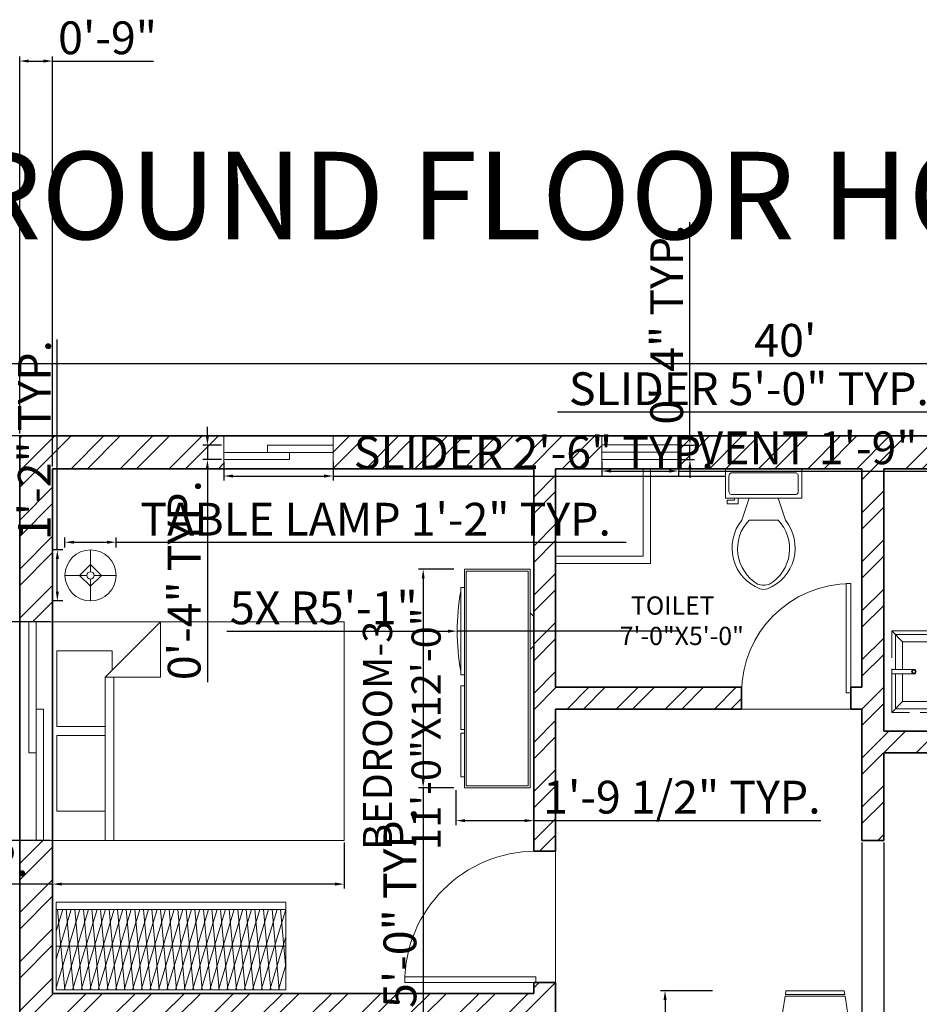
# Model space of a CAD drawing. Units: inches. Extents: x 889 to 1572, y 7262 to 8387.
# Tile 6 of 8: x 1016 to 1263, y 8117 to 8387. Entities that reach past the tile are written whole.
import ezdxf

# ---------------------------------------------------------------- set-up
doc = ezdxf.new("R2010")
doc.units = ezdxf.units.IN
doc.linetypes.add('ACAD_ISO02W100', pattern=[15, 12, -3])
for name, color, linetype, lineweight in [('A-ANNO-DIMS', 2, 'Continuous', 18), ('A-ANNO-TITL', 7, 'Continuous', 35), ('A-AREA-IDEN', 7, 'Continuous', 18), ('A-DOOR', 4, 'Continuous', 18), ('A-FIXT-HIDN', 9, 'ACAD_ISO02W100', 13), ('A-FLOR-FIXT', 9, 'Continuous', 18), ('A-FURN', 8, 'Continuous', 18), ('A-FURN-PATT', 252, 'Continuous', 13), ('A-WALL', 7, 'Continuous', 35), ('A-WALL-PATT', 252, 'Continuous', 13), ('C-SITE', 7, 'Continuous', 30)]:
    doc.layers.add(name, color=color, linetype=linetype, lineweight=lineweight)
doc.layers.add('A-GLAZ', color=244, linetype='Continuous', lineweight=18, true_color=0x991b1e)
doc.styles.get("Standard").update_dxf_attribs({"font": 'arial.ttf'})
doc.dimstyles.new('ISO-25', dxfattribs={"dimtxt": 9, "dimasz": 2.5, "dimexe": 1.25, "dimexo": 0.625, "dimtad": 1, "dimlunit": 3, "dimtxsty": 'Standard', "dimcen": 2.5, "dimadec": 0, "dimazin": 0, "dimtfac": 1, "dimtmove": 0, "dimatfit": 3, "dimfxl": 1, "dimarcsym": 0})

# ---------------------------------------------------------------- blocks, each defined once
blk = doc.blocks.new('*U5')
for p, q in [((-40, 0), (-40, 6)), ((0, 0), (0, 6))]:
    blk.add_line(p, q)
blk.add_lwpolyline([(0, 0), (0, -40), (-1.75, -40), (-1.75, 0)], close=True)
blk.add_arc((0, 0), 40, 180, 270)
blk = doc.blocks.new('*U6')
for p, q in [((0, 0), (0, 6)), ((40, 0), (40, 6))]:
    blk.add_line(p, q)
blk.add_lwpolyline([(0, 0), (0, -40), (1.75, -40), (1.75, 0)], close=True)
blk.add_arc((0, 0), 40, 270, 360)
blk = doc.blocks.new('*U10')
for p, q in [((9.5, -6), (9.5, -2)), ((-8, -8.5), (-8, -8)), ((-7, -8), (-7, -9.5)), ((-4, -8), (-6, -14)), ((4, -8), (6, -14)), ((-10, -8.5), (-8, -8.5)), ((-10, -9.5), (-10, -8.5)), ((-7, -9.5), (-10, -9.5)), ((4, -14), (-4, -14))]:
    blk.add_line(p, q)
blk.add_lwpolyline([(10.5, -8), (10.5, 0), (-10.5, 0), (-10.5, -8)], close=True)
for points in [[(-9.5, -2), (-9.5, -6)], [(8.5, -1), (-8.5, -1)], [(-8.5, -7), (8.5, -7)]]:
    blk.add_lwpolyline(points)
for centre, radius, start, end in [((-8.62, -1.88), 0.884, 81.8699, 188.1301), ((8.62, -1.88), 0.884, 351.8699, 98.1301), ((-8.62, -6.12), 0.884, 171.8699, 278.1301), ((8.62, -6.12), 0.884, 261.8699, 8.1301), ((3.52, -21.58), 12.17, 141.4691, 247.9714), ((4.2, -21.82), 11.33, 136.3677, 238.9468), ((-3.52, -21.58), 12.17, 292.0284, 38.5307), ((-4.2, -21.82), 11.33, 301.053, 43.6321), ((0, -27.88), 4, 245.7318, 294.2682), ((0, -29), 4, 254.8605, 285.1395)]:
    blk.add_arc(centre, radius, start, end)
blk = doc.blocks.new('Bed - Queen')
for p, q in [((0, -80.00003), (0, 0)), ((0, 0), (59.99999, 0)), ((59.99999, 0), (59.99999, -80.00003)), ((7.99999, -1.2), (28.79998, -1.2)), ((7.99999, -14.4), (7.99999, -1.2)), ((28.79998, -1.2), (28.79998, -14.4)), ((31.19999, -1.2), (51.99999, -1.2)), ((31.19999, -14.4), (31.19999, -1.2)), ((51.99999, -1.2), (51.99999, -16.4)), ((0, -14.4), (44.8, -14.4)), ((59.99999, -29.6), (44.8, -14.4)), ((44.8, -14.4), (44.8, -29.6)), ((44.8, -16.8), (0, -16.8)), ((51.99999, -16.4), (46.79936, -16.4)), ((44.8, -29.6), (59.99999, -29.6)), ((59.99999, -80.00003), (0, -80.00003))]:
    blk.add_line(p, q)
blk = doc.blocks.new('Entertainment Center')
for p, q in [((-4, 0), (-5, -1)), ((4, 0), (-4, 0)), ((5, -1), (4, 0)), ((-17, -19), (-17, -1)), ((-17, -1), (43, -1)), ((-16.5, -18.5), (-16.5, -1.5)), ((-16.5, -1.5), (42.5, -1.5)), ((42.5, -1.5), (42.5, -18.5)), ((43, -1), (43, -19)), ((42.5, -18.5), (-16.5, -18.5)), ((43, -19), (-17, -19)), ((-12, -20), (-12, -19)), ((12, -20), (-12, -20)), ((12, -19), (12, -20)), ((15, -20), (15, -19)), ((27, -20), (15, -20)), ((27, -19), (27, -20)), ((28, -20), (28, -19)), ((40, -20), (28, -20)), ((40, -19), (40, -20))]:
    blk.add_line(p, q)
blk.add_arc((0, 40), 61, 259.6111, 280.3889)
blk = doc.blocks.new('Dining Set - 36 x 72 in.')
for p, q in [((-22, 27.5), (-22.1562, 26.50042)), ((-22, 27.5), (-6, 27.5)), ((-5.8437, 26.49966), (-6, 27.5)), ((6, 27.5), (5.8438, 26.50042)), ((6, 27.5), (22, 27.5)), ((22.1563, 26.49966), (22, 27.5)), ((-22.2343, 26.00059), (-23.4847, 17.99762)), ((-22.2304, 26), (-5.7608, 26)), ((-5.8416, 26.5), (-22.1534, 26.5)), ((-4.5152, 17.99762), (-5.7655, 25.99926)), ((5.7657, 26.00059), (4.5153, 17.99762)), ((5.7696, 26), (22.2392, 26)), ((22.1584, 26.5), (5.8466, 26.5)), ((23.4848, 17.99762), (22.2345, 25.99926)), ((36, 18), (-36, 18)), ((-36, 18), (-36, -18)), ((36, -18), (36, 18)), ((-45.5, 8), (-44.5004, 8.15617)), ((-44.5, -8.15843), (-44.5, 8.15338)), ((-44.0006, 8.23428), (-35.9976, 9.48474)), ((-44, 8.23041), (-44, -8.23915)), ((44.0006, 8.23428), (35.9976, 9.48474)), ((44, 8.23041), (44, -8.23915)), ((44.5, -8.15843), (44.5, 8.15338)), ((45.5, 8), (44.5005, 8.15617)), ((-45.5, 8), (-45.5, -8)), ((45.5, 8), (45.5, -8)), ((-44.4997, -8.15631), (-45.5, -8)), ((44.4997, -8.15631), (45.5, -8)), ((-35.9976, -9.48476), (-43.9993, -8.2345)), ((35.9976, -9.48476), (43.9993, -8.2345)), ((-36, -18), (36, -18)), ((-22.2343, -26.0006), (-23.4847, -17.99762)), ((-4.5152, -17.99762), (-5.7655, -25.99928)), ((5.7657, -26.0006), (4.5153, -17.99762)), ((23.4848, -17.99762), (22.2345, -25.99928)), ((-22.2304, -26), (-5.7608, -26)), ((-22, -27.5), (-22.1562, -26.50044)), ((-5.8416, -26.5), (-22.1534, -26.5)), ((-5.8437, -26.49967), (-6, -27.5)), ((5.7696, -26), (22.2392, -26)), ((6, -27.5), (5.8438, -26.50044)), ((22.1584, -26.5), (5.8466, -26.5)), ((22.1563, -26.49967), (22, -27.5)), ((-22, -27.5), (-6, -27.5)), ((6, -27.5), (22, -27.5))]:
    blk.add_line(p, q)
for points in [[(-36, 15), (-31.1772, 14.97754), (-26.8079, 14.91406), (-22.8538, 14.81543), (-19.276, 14.6875), (-16.0362, 14.53613), (-13.0957, 14.36718), (-10.4159, 14.18652), (-7.9583, 14), (-5.6904, 13.81315), (-3.6035, 13.63021), (-1.6954, 13.45508), (0.0365, 13.29166), (1.5945, 13.14388), (2.9811, 13.01562), (4.1988, 12.9108), (5.25, 12.83333), (6.1393, 12.78613), (6.8802, 12.76823), (7.4883, 12.77767), (7.9792, 12.8125), (8.3685, 12.87077), (8.6719, 12.95052), (8.9049, 13.0498), (9.0833, 13.16666), (9.2205, 13.29899), (9.3216, 13.44401), (9.3895, 13.59879), (9.4271, 13.76041), (9.4373, 13.92594), (9.4232, 14.09245), (9.3875, 14.257), (9.3333, 14.41666), (9.2638, 14.56917), (9.1836, 14.71484), (9.0975, 14.85465), (9.0104, 14.98958), (8.9272, 15.1206), (8.8529, 15.2487), (8.7922, 15.37483), (8.75, 15.5), (8.7305, 15.62467), (8.7344, 15.74739), (8.7617, 15.86621), (8.8125, 15.97916), (8.8867, 16.08431), (8.9844, 16.17968), (9.1055, 16.26334), (9.25, 16.33333), (9.4189, 16.38802), (9.6172, 16.42708), (9.8506, 16.45052), (10.125, 16.45833), (10.4463, 16.45052), (10.8203, 16.42708), (11.2529, 16.38802), (11.75, 16.33333), (12.3184, 16.26318), (12.9694, 16.17838), (13.7151, 16.07991), (14.5677, 15.96875), (15.5395, 15.84586), (16.6426, 15.71224), (17.8893, 15.56884), (19.2917, 15.41666), (20.859, 15.25667), (22.5879, 15.08984), (24.4721, 14.91715), (26.5052, 14.73958), (28.6809, 14.5581), (30.9929, 14.3737), (33.4347, 14.18733), (36, 14)], [(-36, 10), (-28.9766, 10.14274), (-23.1725, 10.20442), (-18.4241, 10.19775), (-14.5677, 10.13541), (-11.4399, 10.03011), (-8.877, 9.89453), (-6.7154, 9.74137), (-4.7917, 9.58333), (-2.9698, 9.43082), (-1.2246, 9.28515), (0.4415, 9.14534), (2.026, 9.01041), (3.5266, 8.87939), (4.9408, 8.7513), (6.266, 8.62516), (7.5, 8.5), (8.6411, 8.37549), (9.6914, 8.2539), (10.6538, 8.13818), (11.5312, 8.03125), (12.3267, 7.93603), (13.043, 7.85547), (13.6831, 7.79248), (14.25, 7.75), (14.7471, 7.7303), (15.1797, 7.73307), (15.5537, 7.75732), (15.875, 7.80208), (16.1494, 7.86637), (16.3828, 7.94922), (16.5811, 8.04964), (16.75, 8.16666), (16.8944, 8.29915), (17.0143, 8.44531), (17.1089, 8.60319), (17.1771, 8.77083), (17.218, 8.94629), (17.2305, 9.1276), (17.2137, 9.31282), (17.1667, 9.5), (17.0895, 9.6875), (16.987, 9.875), (16.8649, 10.0625), (16.7292, 10.25), (16.5856, 10.4375), (16.4401, 10.625), (16.2985, 10.8125), (16.1667, 11), (16.05, 11.18733), (15.9518, 11.3737), (15.8752, 11.5581), (15.8229, 11.73958), (15.798, 11.91715), (15.8034, 12.08984), (15.842, 12.25667), (15.9167, 12.41666), (16.0295, 12.56836), (16.1784, 12.70833), (16.3605, 12.83268), (16.5729, 12.9375), (16.8127, 13.01888), (17.0768, 13.07291), (17.3625, 13.0957), (17.6667, 13.08333), (17.9894, 13.03312), (18.3418, 12.94726), (18.7382, 12.82918), (19.1927, 12.68229), (19.7195, 12.51001), (20.3327, 12.31575), (21.0465, 12.10294), (21.875, 11.875), (22.8357, 11.63354), (23.959, 11.37304), (25.2786, 11.08618), (26.8282, 10.76562), (28.6414, 10.40405), (30.752, 9.99414), (33.1936, 9.52856), (36, 9)], [(-36, 5.5), (-30.7157, 5.3348), (-26.069, 5.20963), (-21.9946, 5.11767), (-18.4271, 5.05208), (-15.3009, 5.00602), (-12.5508, 4.97265), (-10.1112, 4.94515), (-7.9167, 4.91666), (-5.909, 4.88167), (-4.0586, 4.83984), (-2.3429, 4.79215), (-0.7396, 4.73958), (0.7739, 4.6831), (2.22, 4.6237), (3.6213, 4.56233), (5, 4.5), (6.373, 4.43782), (7.7344, 4.3776), (9.0723, 4.32129), (10.375, 4.27083), (11.6309, 4.22819), (12.8281, 4.19531), (13.9551, 4.17415), (15, 4.16666), (15.954, 4.17448), (16.819, 4.19791), (17.6001, 4.23698), (18.3021, 4.29166), (18.9299, 4.36198), (19.4883, 4.44791), (19.9823, 4.54948), (20.4167, 4.66666), (20.7969, 4.79899), (21.1302, 4.94401), (21.4245, 5.09879), (21.6875, 5.26041), (21.9271, 5.42594), (22.1511, 5.59245), (22.3672, 5.757), (22.5834, 5.91666), (22.8065, 6.06868), (23.0404, 6.21093), (23.2879, 6.34147), (23.5521, 6.45833), (23.8358, 6.55957), (24.142, 6.64323), (24.4735, 6.70735), (24.8334, 6.75), (25.2235, 6.76969), (25.642, 6.76692), (26.0858, 6.74267), (26.5521, 6.69791), (27.0379, 6.63362), (27.5404, 6.55078), (28.0565, 6.45036), (28.5834, 6.33333), (29.1242, 6.19987), (29.7071, 6.04687), (30.3661, 5.87044), (31.1354, 5.66666), (32.0493, 5.43164), (33.142, 5.16146), (34.4475, 4.85221), (36, 4.5)], [(-36, -1), (-30.7915, -0.6591), (-26.0195, -0.38216), (-21.6519, -0.16284), (-17.6563, 0.00521), (-14.0005, 0.12833), (-10.6523, 0.21289), (-7.5796, 0.26522), (-4.75, 0.29166), (-2.134, 0.29793), (0.2878, 0.28711), (2.5317, 0.26163), (4.6146, 0.22396), (6.5529, 0.17651), (8.3633, 0.12174), (10.0623, 0.06209), (11.6667, 0), (13.1899, -0.06201), (14.6341, -0.1211), (15.9982, -0.17432), (17.2813, -0.21875), (18.4823, -0.25147), (19.6003, -0.26953), (20.6343, -0.27002), (21.5834, -0.25), (22.4481, -0.20768), (23.2357, -0.14584), (23.9549, -0.06836), (24.6146, 0.02083), (25.2235, 0.11784), (25.7904, 0.21875), (26.3241, 0.31966), (26.8334, 0.41666), (27.3265, 0.50618), (27.8099, 0.58593), (28.2894, 0.65397), (28.7709, 0.70833), (29.2601, 0.74707), (29.763, 0.76823), (30.2855, 0.76985), (30.8334, 0.75), (31.4088, 0.70784), (31.9994, 0.64713), (32.589, 0.57275), (33.1615, 0.48958), (33.7008, 0.4025), (34.1908, 0.3164), (34.6153, 0.23616), (34.9584, 0.16666), (35.2099, 0.11165), (35.3848, 0.07031), (35.504, 0.04069), (35.5886, 0.02083), (35.6594, 0.00879), (35.7377, 0.0026), (35.8442, 0.00032), (36, 0)], [(-36, -6.5), (-27.1843, -6.31267), (-20.084, -6.1263), (-14.469, -5.9419), (-10.1094, -5.76042), (-6.7752, -5.58285), (-4.2363, -5.41016), (-2.2629, -5.24333), (-0.625, -5.08334), (0.8708, -4.93099), (2.2715, -4.78646), (3.5872, -4.64974), (4.8281, -4.52084), (6.0046, -4.39974), (7.127, -4.28646), (8.2053, -4.18099), (9.25, -4.08334), (10.2705, -3.99382), (11.2734, -3.91407), (12.2647, -3.84603), (13.25, -3.79167), (14.2354, -3.75293), (15.2266, -3.73177), (16.2295, -3.73015), (17.25, -3.75), (18.2912, -3.79248), (19.3451, -3.85547), (20.4009, -3.93604), (21.4479, -4.03125), (22.4754, -4.13819), (23.4727, -4.25391), (24.4289, -4.37549), (25.3334, -4.5), (26.1785, -4.62492), (26.9694, -4.74935), (27.7145, -4.87281), (28.4219, -4.99479), (29.1, -5.11483), (29.7572, -5.23242), (30.4016, -5.34709), (31.0417, -5.45834), (31.6837, -5.56437), (32.3262, -5.65821), (32.9658, -5.73153), (33.599, -5.77604), (34.2224, -5.78345), (34.8327, -5.74545), (35.4264, -5.65373), (36, -5.5)], [(-36, -10), (-26.4022, -9.81299), (-18.4675, -9.62891), (-11.9839, -9.45069), (-6.7396, -9.28125), (-2.5226, -9.12354), (0.8789, -8.98047), (3.6769, -8.85498), (6.0833, -8.75), (8.2767, -8.66765), (10.3021, -8.60677), (12.1712, -8.56543), (13.8958, -8.54167), (15.4876, -8.53353), (16.9583, -8.53907), (18.3197, -8.55632), (19.5834, -8.58334), (20.7616, -8.61841), (21.8685, -8.66081), (22.9188, -8.71004), (23.9271, -8.76563), (24.9081, -8.82707), (25.8763, -8.89388), (26.8465, -8.96558), (27.8334, -9.04167), (28.8474, -9.12118), (29.8828, -9.20117), (30.93, -9.27824), (31.9792, -9.34896), (33.0205, -9.40991), (34.0443, -9.45768), (35.0407, -9.48885), (36, -9.5)], [(-36, -14.5), (-30.0881, -14.33513), (-25.0332, -14.21224), (-20.7312, -14.12647), (-17.0781, -14.07292), (-13.97, -14.04671), (-11.3027, -14.04297), (-8.9724, -14.05681), (-6.875, -14.08334), (-4.9224, -14.11833), (-3.0905, -14.16016), (-1.3709, -14.20785), (0.2448, -14.26042), (1.7647, -14.3169), (3.1973, -14.3763), (4.5507, -14.43767), (5.8333, -14.5), (7.0554, -14.5621), (8.235, -14.62175), (9.3922, -14.67652), (10.5469, -14.72396), (11.7192, -14.76164), (12.929, -14.78711), (14.1965, -14.79794), (15.5417, -14.79167), (16.9933, -14.76424), (18.6152, -14.70508), (20.4804, -14.60197), (22.6615, -14.44271), (25.2312, -14.21509), (28.2624, -13.9069), (31.8277, -13.50594), (36, -13)]]:
    blk.add_lwpolyline(points)
blk = doc.blocks.new('Lamp - Table')
for p, q in [((0, 7), (0, 1)), ((0, 3), (-3, 0)), ((3, 0), (0, 3)), ((-1, 0), (-7, 0)), ((-3, 0), (0, -3)), ((0, -3), (3, 0)), ((1, 0), (7, 0)), ((0, -1), (0, -7))]:
    blk.add_line(p, q)
for radius in [7, 1]:
    blk.add_circle((0, 0), radius)
blk = doc.blocks.new('*D28')
at = {"layer": 'A-ANNO-DIMS', "color": 0, "lineweight": -2, "transparency": 16777216}
for p, q in [((986.05, 8273.36), (986.05, 8293.82)), ((1466.05, 8273.36), (1466.05, 8293.82)), ((988.55, 8292.57), (1463.55, 8292.57))]:
    blk.add_line(p, q, dxfattribs=at)
at = {"layer": 'A-ANNO-DIMS', "color": 0, "transparency": 16777216}
for points in [[(988.55, 8292.98), (988.55, 8292.15), (986.05, 8292.57)], [(1463.55, 8292.98), (1463.55, 8292.15), (1466.05, 8292.57)]]:
    blk.add_solid(points, dxfattribs=at)
at = {"layer": 'Defpoints', "color": 0, "transparency": 16777216}
for p in [(1466.05, 8292.57), (986.05, 8272.73), (1466.05, 8272.73)]:
    blk.add_point(p, dxfattribs=at)
at = {"layer": 'A-ANNO-DIMS', "color": 0, "transparency": 16777216, "insert": (1226.05, 8297.79), "char_height": 9, "attachment_point": 5}
blk.add_mtext("40'", dxfattribs=at)
blk = doc.blocks.new('GLAZ-VENT-21IN')
for p, q in [((0, 4), (21, 4)), ((0, 2), (21, 2)), ((0, 0), (21, 0))]:
    blk.add_line(p, q)
blk = doc.blocks.new('GLAZ-SLIDER-60IN')
for p, q in [((0, 60), (0, 24)), ((2, 60), (2, 0)), ((2, 36), (4, 36)), ((4, 36), (4, 0)), ((2, 24), (0, 24))]:
    blk.add_line(p, q)
blk = doc.blocks.new('GLAZ-SLIDER-30IN')
for p, q in [((0, 30), (0, 12)), ((2, 30), (2, 0)), ((4, 18), (2, 18)), ((4, 18), (4, 0)), ((2, 12), (0, 12))]:
    blk.add_line(p, q)
blk = doc.blocks.new('*D37')
at = {"layer": 'A-ANNO-DIMS', "color": 0, "lineweight": -2, "transparency": 16777216}
for p, q in [((1271.05, 8270.86), (1271.05, 8280.48)), ((1331.05, 8270.86), (1331.05, 8280.48)), ((1271.05, 8279.23), (1163.57, 8279.23)), ((1328.55, 8279.23), (1273.55, 8279.23))]:
    blk.add_line(p, q, dxfattribs=at)
at = {"layer": 'A-ANNO-DIMS', "color": 0, "transparency": 16777216}
for points in [[(1273.55, 8279.65), (1273.55, 8278.81), (1271.05, 8279.23)], [(1328.55, 8279.65), (1328.55, 8278.81), (1331.05, 8279.23)]]:
    blk.add_solid(points, dxfattribs=at)
at = {"layer": 'Defpoints', "color": 0, "transparency": 16777216}
for p in [(1271.05, 8279.23), (1271.05, 8270.23), (1331.05, 8270.23)]:
    blk.add_point(p, dxfattribs=at)
at = {"layer": 'A-ANNO-DIMS', "color": 0, "transparency": 16777216, "insert": (1216.06, 8284.51), "char_height": 9, "attachment_point": 5}
blk.add_mtext('SLIDER 5\'-0" TYP.', dxfattribs=at)
blk = doc.blocks.new('*D39')
at = {"layer": 'A-ANNO-DIMS', "color": 0, "lineweight": -2, "transparency": 16777216}
for p, q in [((1072.04, 8265.59), (1072.04, 8260.46)), ((1102.04, 8265.59), (1102.04, 8260.46)), ((1074.54, 8261.71), (1099.54, 8261.71)), ((1102.04, 8261.71), (1209.51, 8261.71))]:
    blk.add_line(p, q, dxfattribs=at)
at = {"layer": 'A-ANNO-DIMS', "color": 0, "transparency": 16777216}
for points in [[(1074.54, 8262.13), (1074.54, 8261.29), (1072.04, 8261.71)], [(1099.54, 8262.13), (1099.54, 8261.29), (1102.04, 8261.71)]]:
    blk.add_solid(points, dxfattribs=at)
at = {"layer": 'Defpoints', "color": 0, "transparency": 16777216}
for p in [(1072.04, 8266.21), (1102.04, 8266.21), (1102.04, 8261.71)]:
    blk.add_point(p, dxfattribs=at)
at = {"layer": 'A-ANNO-DIMS', "color": 0, "transparency": 16777216, "insert": (1157.03, 8266.99), "char_height": 9, "attachment_point": 5}
blk.add_mtext('SLIDER 2\'-6" TYP.', dxfattribs=at)
blk = doc.blocks.new('*D40')
at = {"layer": 'A-ANNO-DIMS', "color": 0, "lineweight": -2, "transparency": 16777216}
for p, q in [((1067.54, 8272.71), (1067.54, 8275.21)), ((1071.41, 8270.21), (1066.29, 8270.21)), ((1067.54, 8270.21), (1067.54, 8266.21)), ((1071.41, 8266.21), (1066.29, 8266.21)), ((1067.54, 8263.71), (1067.54, 8205.1))]:
    blk.add_line(p, q, dxfattribs=at)
at = {"layer": 'A-ANNO-DIMS', "color": 0, "transparency": 16777216}
for points in [[(1067.12, 8272.71), (1067.95, 8272.71), (1067.54, 8270.21)], [(1067.12, 8263.71), (1067.95, 8263.71), (1067.54, 8266.21)]]:
    blk.add_solid(points, dxfattribs=at)
at = {"layer": 'Defpoints', "color": 0, "transparency": 16777216}
for p in [(1072.04, 8270.21), (1067.54, 8266.21), (1072.04, 8266.21)]:
    blk.add_point(p, dxfattribs=at)
at = {"layer": 'A-ANNO-DIMS', "color": 0, "transparency": 16777216, "insert": (1062.32, 8233.16), "char_height": 9, "attachment_point": 5, "rotation": 90}
blk.add_mtext('0\'-4" TYP.', dxfattribs=at)
blk = doc.blocks.new('*D41')
at = {"layer": 'A-ANNO-DIMS', "color": 0, "lineweight": -2, "transparency": 16777216}
for p, q in [((1175.74, 8265.61), (1175.74, 8261.83)), ((1196.74, 8265.61), (1196.74, 8261.83)), ((1178.24, 8263.08), (1194.24, 8263.08)), ((1196.74, 8263.08), (1292.84, 8263.08))]:
    blk.add_line(p, q, dxfattribs=at)
at = {"layer": 'A-ANNO-DIMS', "color": 0, "transparency": 16777216}
for points in [[(1178.24, 8263.5), (1178.24, 8262.66), (1175.74, 8263.08)], [(1194.24, 8263.5), (1194.24, 8262.66), (1196.74, 8263.08)]]:
    blk.add_solid(points, dxfattribs=at)
at = {"layer": 'Defpoints', "color": 0, "transparency": 16777216}
for p in [(1175.74, 8266.23), (1196.74, 8266.23), (1196.74, 8263.08)]:
    blk.add_point(p, dxfattribs=at)
at = {"layer": 'A-ANNO-DIMS', "color": 0, "transparency": 16777216, "insert": (1246.04, 8268.3), "char_height": 9, "attachment_point": 5}
blk.add_mtext('VENT 1\'-9" TYP.', dxfattribs=at)
blk = doc.blocks.new('*D42')
at = {"layer": 'A-ANNO-DIMS', "color": 0, "lineweight": -2, "transparency": 16777216}
for p, q in [((1199.89, 8272.73), (1199.89, 8331.34)), ((1197.36, 8270.23), (1201.14, 8270.23)), ((1199.89, 8266.23), (1199.89, 8270.23)), ((1197.36, 8266.23), (1201.14, 8266.23)), ((1199.89, 8263.73), (1199.89, 8261.23))]:
    blk.add_line(p, q, dxfattribs=at)
at = {"layer": 'A-ANNO-DIMS', "color": 0, "transparency": 16777216}
for points in [[(1199.47, 8272.73), (1200.3, 8272.73), (1199.89, 8270.23)], [(1199.47, 8263.73), (1200.3, 8263.73), (1199.89, 8266.23)]]:
    blk.add_solid(points, dxfattribs=at)
at = {"layer": 'Defpoints', "color": 0, "transparency": 16777216}
for p in [(1196.74, 8270.23), (1199.89, 8270.23), (1196.74, 8266.23)]:
    blk.add_point(p, dxfattribs=at)
at = {"layer": 'A-ANNO-DIMS', "color": 0, "transparency": 16777216, "insert": (1194.67, 8303.29), "char_height": 9, "attachment_point": 5, "rotation": 90}
blk.add_mtext('0\'-4" TYP.', dxfattribs=at)
blk = doc.blocks.new('*D43')
at = {"layer": 'A-ANNO-DIMS', "color": 0, "lineweight": -2, "transparency": 16777216}
for p, q in [((1025.05, 8161.11), (1025.05, 8148.48)), ((1105.05, 8161.11), (1105.05, 8148.48)), ((1025.05, 8149.73), (888.91, 8149.73)), ((1102.55, 8149.73), (1027.55, 8149.73))]:
    blk.add_line(p, q, dxfattribs=at)
at = {"layer": 'A-ANNO-DIMS', "color": 0, "transparency": 16777216}
for points in [[(1027.55, 8150.15), (1027.55, 8149.31), (1025.05, 8149.73)], [(1102.55, 8150.15), (1102.55, 8149.31), (1105.05, 8149.73)]]:
    blk.add_solid(points, dxfattribs=at)
at = {"layer": 'Defpoints', "color": 0, "transparency": 16777216}
for p in [(1025.05, 8161.73), (1105.05, 8161.73), (1025.05, 8149.73)]:
    blk.add_point(p, dxfattribs=at)
at = {"layer": 'A-ANNO-DIMS', "color": 0, "transparency": 16777216, "insert": (955.73, 8155.29), "char_height": 9, "attachment_point": 5}
blk.add_mtext('QUEEN BED 6\'-8" TYP.', dxfattribs=at)
blk = doc.blocks.new('*D44')
at = {"layer": 'A-ANNO-DIMS', "color": 0, "lineweight": -2, "transparency": 16777216}
for p, q in [((1024.42, 8221.73), (1011.8, 8221.73)), ((1013.05, 8164.23), (1013.05, 8219.23)), ((1024.42, 8161.73), (1011.8, 8161.73))]:
    blk.add_line(p, q, dxfattribs=at)
at = {"layer": 'A-ANNO-DIMS', "color": 0, "transparency": 16777216}
for points in [[(1012.63, 8219.23), (1013.47, 8219.23), (1013.05, 8221.73)], [(1012.63, 8164.23), (1013.47, 8164.23), (1013.05, 8161.73)]]:
    blk.add_solid(points, dxfattribs=at)
at = {"layer": 'Defpoints', "color": 0, "transparency": 16777216}
for p in [(1013.05, 8221.73), (1025.05, 8221.73), (1025.05, 8161.73)]:
    blk.add_point(p, dxfattribs=at)
at = {"layer": 'A-ANNO-DIMS', "color": 0, "transparency": 16777216, "insert": (1007.83, 8191.73), "char_height": 9, "attachment_point": 5, "rotation": 90}
blk.add_mtext('5\'-0" TYP.', dxfattribs=at)
blk = doc.blocks.new('*D45')
at = {"layer": 'A-ANNO-DIMS', "color": 0, "lineweight": -2, "transparency": 16777216}
for p, q in [((1135.09, 8236.14), (1125.47, 8236.14)), ((1126.72, 8233.64), (1126.72, 8178.64)), ((1135.09, 8176.14), (1125.47, 8176.14)), ((1126.72, 8176.14), (1126.72, 8041.81))]:
    blk.add_line(p, q, dxfattribs=at)
at = {"layer": 'A-ANNO-DIMS', "color": 0, "transparency": 16777216}
for points in [[(1126.3, 8233.64), (1127.13, 8233.64), (1126.72, 8236.14)], [(1126.3, 8178.64), (1127.13, 8178.64), (1126.72, 8176.14)]]:
    blk.add_solid(points, dxfattribs=at)
at = {"layer": 'Defpoints', "color": 0, "transparency": 16777216}
for p in [(1135.72, 8236.14), (1126.72, 8176.14), (1135.72, 8176.14)]:
    blk.add_point(p, dxfattribs=at)
at = {"layer": 'A-ANNO-DIMS', "color": 0, "transparency": 16777216, "insert": (1121.5, 8107.73), "char_height": 9, "attachment_point": 5, "rotation": 90}
blk.add_mtext('MEDIA UNIT 5\'-0" TYP.', dxfattribs=at)
blk = doc.blocks.new('*D46')
at = {"layer": 'A-ANNO-DIMS', "color": 0, "lineweight": -2, "transparency": 16777216}
for p, q in [((1135.72, 8175.52), (1135.72, 8165.89)), ((1157.05, 8175.52), (1157.05, 8165.89)), ((1138.22, 8167.14), (1154.55, 8167.14)), ((1157.05, 8167.14), (1235.78, 8167.14))]:
    blk.add_line(p, q, dxfattribs=at)
at = {"layer": 'A-ANNO-DIMS', "color": 0, "transparency": 16777216}
for points in [[(1138.22, 8167.56), (1138.22, 8166.73), (1135.72, 8167.14)], [(1154.55, 8167.56), (1154.55, 8166.73), (1157.05, 8167.14)]]:
    blk.add_solid(points, dxfattribs=at)
at = {"layer": 'Defpoints', "color": 0, "transparency": 16777216}
for p in [(1135.72, 8176.14), (1157.05, 8176.14), (1157.05, 8167.14)]:
    blk.add_point(p, dxfattribs=at)
at = {"layer": 'A-ANNO-DIMS', "color": 0, "transparency": 16777216, "insert": (1197.67, 8172.42), "char_height": 9, "attachment_point": 5}
blk.add_mtext('1\'-9 1/2" TYP.', dxfattribs=at)
blk = doc.blocks.new('*D53')
at = {"layer": 'A-ANNO-DIMS', "color": 0, "lineweight": -2, "transparency": 16777216}
for p, q in [((1028.47, 8242.08), (1028.47, 8244.8)), ((1042.47, 8242.08), (1042.47, 8244.8)), ((1030.97, 8243.55), (1039.97, 8243.55)), ((1042.47, 8243.55), (1182.37, 8243.55))]:
    blk.add_line(p, q, dxfattribs=at)
at = {"layer": 'A-ANNO-DIMS', "color": 0, "transparency": 16777216}
for points in [[(1030.97, 8243.97), (1030.97, 8243.14), (1028.47, 8243.55)], [(1039.97, 8243.97), (1039.97, 8243.14), (1042.47, 8243.55)]]:
    blk.add_solid(points, dxfattribs=at)
at = {"layer": 'Defpoints', "color": 0, "transparency": 16777216}
for p in [(1042.47, 8243.55), (1028.47, 8241.45), (1042.47, 8241.45)]:
    blk.add_point(p, dxfattribs=at)
at = {"layer": 'A-ANNO-DIMS', "color": 0, "transparency": 16777216, "insert": (1113.67, 8248.7), "char_height": 9, "attachment_point": 5}
blk.add_mtext('TABLE LAMP 1\'-2" TYP.', dxfattribs=at)
blk = doc.blocks.new('*D54')
at = {"layer": 'A-ANNO-DIMS', "color": 0, "lineweight": -2, "transparency": 16777216}
for p, q in [((1026.37, 8241.45), (1026.37, 8299.22)), ((1027.85, 8241.45), (1025.12, 8241.45)), ((1026.37, 8229.95), (1026.37, 8238.95)), ((1027.85, 8227.45), (1025.12, 8227.45))]:
    blk.add_line(p, q, dxfattribs=at)
at = {"layer": 'A-ANNO-DIMS', "color": 0, "transparency": 16777216}
for points in [[(1025.96, 8238.95), (1026.79, 8238.95), (1026.37, 8241.45)], [(1025.96, 8229.95), (1026.79, 8229.95), (1026.37, 8227.45)]]:
    blk.add_solid(points, dxfattribs=at)
at = {"layer": 'Defpoints', "color": 0, "transparency": 16777216}
for p in [(1026.37, 8241.45), (1028.47, 8241.45), (1028.47, 8227.45)]:
    blk.add_point(p, dxfattribs=at)
at = {"layer": 'A-ANNO-DIMS', "color": 0, "transparency": 16777216, "insert": (1021.23, 8271.58), "char_height": 9, "attachment_point": 5, "rotation": 90}
blk.add_mtext('1\'-2" TYP.', dxfattribs=at)
blk = doc.blocks.new('*D65')
at = {"layer": 'A-ANNO-DIMS', "color": 0, "lineweight": -2, "transparency": 16777216}
for p, q in [((1206.09, 8120.44), (1191.81, 8120.44)), ((1193.06, 8117.94), (1193.06, 8031.94)), ((1206.09, 8029.44), (1191.81, 8029.44)), ((1193.06, 8029.44), (1193.06, 7926.77))]:
    blk.add_line(p, q, dxfattribs=at)
at = {"layer": 'A-ANNO-DIMS', "color": 0, "transparency": 16777216}
for points in [[(1192.64, 8117.94), (1193.48, 8117.94), (1193.06, 8120.44)], [(1192.64, 8031.94), (1193.48, 8031.94), (1193.06, 8029.44)]]:
    blk.add_solid(points, dxfattribs=at)
at = {"layer": 'Defpoints', "color": 0, "transparency": 16777216}
for p in [(1206.71, 8120.44), (1193.06, 8029.44), (1206.71, 8029.44)]:
    blk.add_point(p, dxfattribs=at)
at = {"layer": 'A-ANNO-DIMS', "color": 0, "transparency": 16777216, "insert": (1187.78, 7976.85), "char_height": 9, "attachment_point": 5, "rotation": 90}
blk.add_mtext('DINING SET 7\'-7"', dxfattribs=at)
blk = doc.blocks.new('*D73')
at = {"layer": 'A-ANNO-DIMS', "color": 0, "lineweight": -2, "transparency": 16777216}
for p, q in [((1016.05, 8273.36), (1016.05, 8376.85)), ((1018.55, 8375.6), (1022.55, 8375.6)), ((1025.05, 8264.36), (1025.05, 8376.85)), ((1025.05, 8375.6), (1052.72, 8375.6))]:
    blk.add_line(p, q, dxfattribs=at)
at = {"layer": 'A-ANNO-DIMS', "color": 0, "transparency": 16777216}
for points in [[(1018.55, 8376.02), (1018.55, 8375.18), (1016.05, 8375.6)], [(1022.55, 8376.02), (1022.55, 8375.18), (1025.05, 8375.6)]]:
    blk.add_solid(points, dxfattribs=at)
at = {"layer": 'Defpoints', "color": 0, "transparency": 16777216}
for p in [(1025.05, 8375.6), (1016.05, 8272.73), (1025.05, 8263.73)]:
    blk.add_point(p, dxfattribs=at)
at = {"layer": 'A-ANNO-DIMS', "color": 0, "transparency": 16777216, "insert": (1040.14, 8380.82), "char_height": 9, "attachment_point": 5}
blk.add_mtext('0\'-9"', dxfattribs=at)
blk = doc.blocks.new('*D74')
at = {"layer": 'A-ANNO-DIMS', "color": 0, "lineweight": -2, "transparency": 16777216}
for p, q in [((1247.05, 8161.11), (1247.05, 7262.35)), ((1253.05, 8161.11), (1253.05, 7262.35)), ((1244.55, 7263.6), (1242.05, 7263.6)), ((1247.05, 7263.6), (1253.05, 7263.6)), ((1255.55, 7263.6), (1283.22, 7263.6))]:
    blk.add_line(p, q, dxfattribs=at)
at = {"layer": 'A-ANNO-DIMS', "color": 0, "transparency": 16777216}
for points in [[(1244.55, 7264.02), (1244.55, 7263.19), (1247.05, 7263.6)], [(1255.55, 7264.02), (1255.55, 7263.19), (1253.05, 7263.6)]]:
    blk.add_solid(points, dxfattribs=at)
at = {"layer": 'Defpoints', "color": 0, "transparency": 16777216}
for p in [(1247.05, 8161.73), (1253.05, 8161.73), (1253.05, 7263.6)]:
    blk.add_point(p, dxfattribs=at)
at = {"layer": 'A-ANNO-DIMS', "color": 0, "transparency": 16777216, "insert": (1270.64, 7268.82), "char_height": 9, "attachment_point": 5}
blk.add_mtext('0\'-6"', dxfattribs=at)
blk = doc.blocks.new('*D79')
at = {"layer": 'A-ANNO-DIMS', "color": 0, "lineweight": -2, "transparency": 16777216}
for p, q in [((1072.89, 8219.14), (1133.55, 8219.14)), ((1197.05, 8219.14), (1136.05, 8219.14))]:
    blk.add_line(p, q, dxfattribs=at)
at = {"layer": 'A-ANNO-DIMS', "color": 0, "transparency": 16777216}
blk.add_solid([(1133.55, 8219.56), (1133.55, 8218.73), (1136.05, 8219.14)], dxfattribs=at)
at = {"layer": 'Defpoints', "color": 0, "transparency": 16777216}
for p in [(1136.05, 8219.14), (1197.05, 8219.14)]:
    blk.add_point(p, dxfattribs=at)
at = {"layer": 'A-ANNO-DIMS', "color": 0, "transparency": 16777216, "insert": (1099.45, 8224.37), "char_height": 9, "attachment_point": 5}
blk.add_mtext('5X R5\'-1"', dxfattribs=at)

msp = doc.modelspace()

# ---------------------------------------------------------------- hatches: boundary and pattern name
at = {"layer": 'A-FURN-PATT'}
h = msp.add_hatch(dxfattribs=at)
h.set_pattern_fill('ANSI31', color=256, scale=0.7085884, angle=28.05249, style=0)
h.paths.add_polyline_path([(1026.049, 8120.731), (1089.076, 8120.731), (1089.076, 8142.731), (1026.049, 8142.731)])
h = msp.add_hatch(dxfattribs=at)
h.set_pattern_fill('ANSI31', color=256, scale=0.7377319, angle=50.20848, style=0)
h.paths.add_polyline_path([(1026.049, 8120.731), (1089.076, 8120.731), (1089.076, 8142.731), (1026.049, 8142.731)])
at = {"layer": 'A-WALL-PATT'}
h = msp.add_hatch(dxfattribs=at)
h.set_pattern_fill('ANSI32', color=256)
h.paths.add_polyline_path([(1166.049, 7624.731), (1163.049, 7624.731), (1163.049, 7774.731), (1154.049, 7774.731), (1154.049, 7768.731), (1157.049, 7768.731), (1157.049, 7624.731), (1106.049, 7624.731), (1106.049, 7615.731), (1166.049, 7615.731), (1166.049, 7618.431)])
h.paths.add_polyline_path([(1025.049, 7666.731), (1016.049, 7666.731), (1016.049, 7615.731), (1076.049, 7615.731), (1076.049, 7624.731), (1025.049, 7624.731)])
h.paths.add_polyline_path([(1025.049, 7768.731), (1118.049, 7768.731), (1118.049, 7774.731), (1025.049, 7774.731), (1025.049, 7897.731), (1115.049, 7897.731), (1115.049, 7906.731), (1109.049, 7906.731), (1109.049, 7903.731), (1025.049, 7903.731), (1025.049, 7923.231), (1016.049, 7923.231), (1016.049, 7726.731), (1025.049, 7726.731)])
h.paths.add_polyline_path([(1436.049, 7897.731), (1427.049, 7897.731), (1427.049, 7883.374), (1436.049, 7883.374)])
h.paths.add_polyline_path([(1436.049, 7853.374), (1427.049, 7853.374), (1427.049, 7843.731), (1415.049, 7843.731), (1415.049, 7837.731), (1427.049, 7837.731), (1427.049, 7831.731), (1436.049, 7831.731)])
h.paths.add_polyline_path([(1436.049, 8010.183), (1427.049, 8010.183), (1427.049, 7970.456), (1370.049, 7970.456), (1370.049, 7963.731), (1427.049, 7963.731), (1427.049, 7957.731), (1436.049, 7957.731)])
h.paths.add_polyline_path([(1436.049, 7747.731), (1427.049, 7747.731), (1427.049, 7741.731), (1344.721, 7741.731), (1344.721, 7735.731), (1349.049, 7735.731), (1349.049, 7672.731), (1355.049, 7672.731), (1355.049, 7735.731), (1427.049, 7735.731), (1427.049, 7721.931), (1436.049, 7721.931)])
h.paths.add_polyline_path([(1436.049, 7700.931), (1427.049, 7700.931), (1427.049, 7591.731), (1355.049, 7591.731), (1355.049, 7642.731), (1349.049, 7642.731), (1349.049, 7591.731), (1310.049, 7591.731), (1310.049, 7582.731), (1436.049, 7582.731)])
h.paths.add_polyline_path([(1392.42, 8272.731), (1331.049, 8272.731), (1331.049, 8263.731), (1349.049, 8263.731), (1349.049, 8224.731), (1355.049, 8224.731), (1355.049, 8263.731), (1392.42, 8263.731)])
h.paths.add_polyline_path([(1271.049, 8272.731), (1196.736, 8272.731), (1196.736, 8263.731), (1247.049, 8263.731), (1247.049, 8203.731), (1244.049, 8203.731), (1244.049, 8197.731), (1247.049, 8197.731), (1247.049, 8161.731), (1253.049, 8161.731), (1253.049, 8185.731), (1295.049, 8185.731), (1295.049, 8191.731), (1253.049, 8191.731), (1253.049, 8263.731), (1271.049, 8263.731)])
h.paths.add_polyline_path([(1175.736, 8272.731), (1102.037, 8272.731), (1102.037, 8263.731), (1157.049, 8263.731), (1157.049, 8158.731), (1163.049, 8158.731), (1163.049, 8197.731), (1214.049, 8197.731), (1214.049, 8203.731), (1163.049, 8203.731), (1163.049, 8263.731), (1175.736, 8263.731)])
h.paths.add_polyline_path([(1072.037, 8272.731), (1016.049, 8272.731), (1016.049, 8221.731), (1025.049, 8221.731), (1025.049, 8263.731), (1072.037, 8263.731)])
h.paths.add_polyline_path([(1163.049, 8122.731), (1157.049, 8122.731), (1157.049, 8119.731), (1025.049, 8119.731), (1025.049, 8161.731), (1016.049, 8161.731), (1016.049, 8071.731), (1025.049, 8071.731), (1025.049, 8113.731), (1157.049, 8113.731), (1157.049, 8110.731), (1163.049, 8110.731)])
h.paths.add_polyline_path([(1025.049, 8011.731), (1016.049, 8011.731), (1016.049, 7944.231), (1025.049, 7944.231), (1025.049, 7963.731), (1109.049, 7963.731), (1109.049, 7936.731), (1115.049, 7936.731), (1115.049, 7963.731), (1163.049, 7963.731), (1163.049, 8074.731), (1157.049, 8074.731), (1157.049, 7969.731), (1025.049, 7969.731)])
h.paths.add_polyline_path([(1314.721, 7741.731), (1307.049, 7741.731), (1307.049, 7837.731), (1319.049, 7837.731), (1319.049, 7843.731), (1307.049, 7843.731), (1307.049, 7963.731), (1310.049, 7963.731), (1310.049, 7970.456), (1301.049, 7970.456), (1301.049, 7837.731), (1301.049, 7741.731), (1250.049, 7741.731), (1250.049, 7735.731), (1314.721, 7735.731)])
h.paths.add_polyline_path([(1211.049, 7735.731), (1214.049, 7735.731), (1214.049, 7741.731), (1205.049, 7741.731), (1205.049, 7624.731), (1202.049, 7624.731), (1202.049, 7615.731), (1205.049, 7615.731), (1205.049, 7582.731), (1250.049, 7582.731), (1250.049, 7591.731), (1211.049, 7591.731)])
h.paths.add_polyline_path([(1436.049, 8260.718), (1427.049, 8260.718), (1427.049, 8191.731), (1355.049, 8191.731), (1355.049, 8194.731), (1349.049, 8194.731), (1349.049, 8191.731), (1343.049, 8191.731), (1343.049, 8185.731), (1427.049, 8185.731), (1427.049, 8070.183), (1436.049, 8070.183)])

# ---------------------------------------------------------------- linework, layer by layer
at = {"layer": 'A-DOOR'}
for p, q in [((1244.049, 8197.731), (1214.049, 8197.731)), ((1163.049, 8158.731), (1163.049, 8122.731))]:
    msp.add_line(p, q, dxfattribs=at)
at = {"layer": 'A-FIXT-HIDN'}
msp.add_lwpolyline([(1255.235, 8219.196), (1275.072, 8219.196), (1275.072, 8196.835), (1255.235, 8196.835)], close=True, dxfattribs=at)
at = {"layer": 'A-FLOR-FIXT'}
for p, q in [((1187.049, 8263.731), (1187.049, 8239.731)), ((1189.049, 8263.731), (1189.049, 8237.731)), ((1163.049, 8239.731), (1187.049, 8239.731)), ((1163.049, 8237.731), (1189.049, 8237.731)), ((1258.235, 8216.196), (1255.235, 8219.196)), ((1255.235, 8208.616), (1261.113, 8208.616)), ((1255.235, 8207.416), (1261.113, 8207.416)), ((1258.235, 8199.835), (1255.235, 8196.835))]:
    msp.add_line(p, q, dxfattribs=at)
for points in [[(1256.235, 8208.616), (1256.235, 8218.196), (1274.072, 8218.196), (1274.072, 8197.835), (1256.235, 8197.835), (1256.235, 8207.416)], [(1258.235, 8208.616), (1258.235, 8216.196), (1272.072, 8216.196), (1272.072, 8199.835), (1258.235, 8199.835), (1258.235, 8207.416)]]:
    msp.add_lwpolyline(points, dxfattribs=at)
for radius in [0.631, 0.431]:
    msp.add_circle((1261.309, 8208.016), radius, dxfattribs=at)
at = {"layer": 'A-FURN'}
for p, q in [((1026.049, 8144.731), (1089.076, 8144.731)), ((1026.049, 8144.731), (1026.049, 8120.731)), ((1089.076, 8144.731), (1089.076, 8120.731)), ((1026.049, 8142.731), (1089.076, 8142.731)), ((1026.049, 8132.731), (1089.076, 8132.731)), ((1026.049, 8120.731), (1089.076, 8120.731))]:
    msp.add_line(p, q, dxfattribs=at)
at = {"layer": 'A-GLAZ'}
for points in [[(1102.037, 8263.731), (1072.037, 8263.731), (1072.037, 8272.731), (1102.037, 8272.731)], [(1175.736, 8272.731), (1196.736, 8272.731), (1196.736, 8263.731), (1175.736, 8263.731)], [(1016.049, 8221.731), (1025.049, 8221.731), (1025.049, 8161.731), (1016.049, 8161.731)]]:
    msp.add_lwpolyline(points, close=True, dxfattribs=at)
at = {"layer": 'A-WALL'}
for p, q in [((1016.049, 8272.731), (1016.049, 7393.731)), ((1016.049, 8272.731), (1392.42, 8272.731)), ((1025.049, 8263.731), (1157.049, 8263.731)), ((1025.049, 8263.731), (1025.049, 8119.731)), ((1157.049, 8263.731), (1157.049, 8158.731)), ((1163.049, 8263.731), (1163.049, 8203.731)), ((1163.049, 8263.731), (1247.049, 8263.731)), ((1247.049, 8263.731), (1247.049, 8203.731)), ((1253.049, 8263.731), (1253.049, 8191.731)), ((1253.049, 8263.731), (1349.049, 8263.731)), ((1163.049, 8203.731), (1214.049, 8203.731)), ((1214.049, 8197.731), (1214.049, 8203.731)), ((1244.049, 8197.731), (1244.049, 8203.731)), ((1244.049, 8203.731), (1247.049, 8203.731)), ((1163.049, 8197.731), (1214.049, 8197.731)), ((1163.049, 8197.731), (1163.049, 8158.731)), ((1244.049, 8197.731), (1247.049, 8197.731)), ((1247.049, 8197.731), (1247.049, 8161.731)), ((1253.049, 8191.731), (1295.049, 8191.731)), ((1253.049, 8185.731), (1295.049, 8185.731)), ((1253.049, 8185.731), (1253.049, 8161.731)), ((1247.049, 8161.731), (1253.049, 8161.731)), ((1157.049, 8158.731), (1163.049, 8158.731)), ((1157.049, 8122.731), (1163.049, 8122.731)), ((1157.049, 8122.731), (1157.049, 8119.731)), ((1163.049, 8122.731), (1163.049, 8110.731)), ((1025.049, 8119.731), (1157.049, 8119.731))]:
    msp.add_line(p, q, dxfattribs=at)
at = {"layer": 'C-SITE'}
msp.add_line((1016.049, 8272.731), (986.049, 8272.731), dxfattribs=at)

# ---------------------------------------------------------------- block references
at = {"layer": 'A-DOOR'}
for name, p, xscale, yscale, zscale, rotation in [('*U6', (1244.049, 8202.231), 0.75, 0.75, 0.75, 180.0000000000077), ('*U5', (1157.649, 8122.731), 0.9, 0.9, 0.9, 270.0000000000003)]:
    msp.add_blockref(name, p, dxfattribs=dict(at, xscale=xscale, yscale=yscale, zscale=zscale, rotation=rotation))
at = {"layer": 'A-FLOR-FIXT'}
msp.add_blockref('*U10', (1220.099, 8263.6), dxfattribs=at)
at = {"layer": 'A-FURN'}
msp.add_blockref('Lamp - Table', (1035.473, 8234.453), dxfattribs=at)
for name, p, rotation in [('Entertainment Center', (1157.049, 8219.145), 270), ('Bed - Queen', (1025.049, 8161.731), 90), ('Dining Set - 36 x 72 in.', (1234.21, 8074.936), 270)]:
    msp.add_blockref(name, p, dxfattribs=dict(at, rotation=rotation))
at = {"layer": 'A-GLAZ', "rotation": 269.9999999999928}
msp.add_blockref('GLAZ-SLIDER-30IN', (1072.038, 8270.211), dxfattribs=at)
at = {"layer": 'A-GLAZ'}
for name, p in [('GLAZ-VENT-21IN', (1175.736, 8266.231)), ('GLAZ-SLIDER-60IN', (1018.549, 8161.731))]:
    msp.add_blockref(name, p, dxfattribs=at)

# ---------------------------------------------------------------- texts
at = {"layer": 'A-ANNO-TITL', "insert": (978.629, 8350.694), "char_height": 24, "attachment_point": 1}
msp.add_mtext_dynamic_manual_height_columns('GROUND FLOOR HOUSE PLAN', width=625.16453, gutter_width=0, heights=[25.177], dxfattribs=at)
at = {"layer": 'A-AREA-IDEN', "insert": (1180.637, 8228.669), "char_height": 5, "attachment_point": 1}
msp.add_mtext_dynamic_manual_height_columns('  TOILET\\P7\'-0"X5\'-0"', width=32.40356, gutter_width=12.5, heights=[0], dxfattribs=at)
at = {"layer": 'A-AREA-IDEN', "insert": (1110.185, 8159.067), "char_height": 8, "attachment_point": 1, "rotation": 90}
msp.add_mtext_dynamic_manual_height_columns('BEDROOM-3\\P11\'-0"X12\'-0"', width=66.55508, gutter_width=12.5, heights=[0], dxfattribs=at)

# ---------------------------------------------------------------- dimensions: what is measured, and where the dimension line sits
at = {"layer": 'A-ANNO-DIMS'}
for base, p1, p2, override, picture, middle in [((1025.049, 8375.6), (1016.049, 8272.731), (1025.049, 8263.731), {"dimdec": 1, "dimlfac": 1, "dimrnd": 0, "dimzin": 1, "dimdsep": 46, "dimlunit": 4, "dimfrac": 2}, '*D73', (1040.136, 8380.82)), ((1466.049, 8292.566), (986.049, 8272.731), (1466.049, 8272.731), {"dimclrd": 0, "dimclre": 0, "dimclrt": 0}, '*D28', (1226.049, 8297.786)), ((1253.049, 7263.604), (1247.049, 8161.731), (1253.049, 8161.731), {"dimdec": 1, "dimlfac": 1, "dimrnd": 0, "dimzin": 1, "dimdsep": 46, "dimlunit": 4, "dimfrac": 2}, '*D74', (1270.636, 7268.824))]:
    dim = msp.add_linear_dim(base=base, p1=p1, p2=p2, dimstyle='ISO-25', override=override, dxfattribs=at)
    dim.commit()
    dim.dimension.update_dxf_attribs({"geometry": picture, "text_midpoint": middle})
for base, p1, p2, angle, text, picture, middle in [((1199.886, 8270.231), (1196.736, 8266.231), (1196.736, 8270.231), 90, '<> TYP.', '*D42', (1194.666, 8303.286)), ((1271.049, 8279.231), (1331.049, 8270.231), (1271.049, 8270.231), 180, 'SLIDER <> TYP.', '*D37', (1216.06, 8284.51)), ((1026.373, 8241.453), (1028.473, 8227.453), (1028.473, 8241.453), 90, '<> TYP.', '*D54', (1021.227, 8271.585)), ((1067.537, 8266.211), (1072.037, 8270.211), (1072.037, 8266.211), 270, '<> TYP.', '*D40', (1062.317, 8233.156)), ((1126.715, 8176.145), (1135.715, 8236.145), (1135.715, 8176.145), 270, 'MEDIA UNIT <> TYP.', '*D45', (1121.495, 8107.727)), ((1013.049, 8221.731), (1025.049, 8161.731), (1025.049, 8221.731), 90, '<> TYP.', '*D44', (1007.828, 8191.731)), ((1025.049, 8149.731), (1105.049, 8161.731), (1025.049, 8161.731), 180, 'QUEEN BED <> TYP.', '*D43', (955.728, 8155.286)), ((1193.06, 8029.436), (1206.71, 8120.436), (1206.71, 8029.436), 270, 'DINING SET <>', '*D65', (1187.782, 7976.85))]:
    dim = msp.add_linear_dim(base=base, p1=p1, p2=p2, angle=angle, text=text, dimstyle='ISO-25', override={"dimdec": 1, "dimlfac": 1, "dimrnd": 0, "dimzin": 1, "dimdsep": 46, "dimlunit": 4, "dimfrac": 2}, dxfattribs=at)
    dim.commit()
    dim.dimension.update_dxf_attribs({"geometry": picture, "text_midpoint": middle})
for base, p1, p2, text, picture, middle in [((1102.037, 8261.711), (1072.037, 8266.211), (1102.037, 8266.211), 'SLIDER <> TYP.', '*D39', (1157.026, 8266.989)), ((1196.736, 8263.081), (1175.736, 8266.231), (1196.736, 8266.231), 'VENT <> TYP.', '*D41', (1246.037, 8268.301)), ((1042.473, 8243.553), (1028.473, 8241.453), (1042.473, 8241.453), 'TABLE LAMP <> TYP.', '*D53', (1113.669, 8248.7)), ((1157.049, 8167.145), (1135.715, 8176.145), (1157.049, 8176.145), '<> TYP.', '*D46', (1197.665, 8172.423))]:
    dim = msp.add_linear_dim(base=base, p1=p1, p2=p2, text=text, dimstyle='ISO-25', override={"dimdec": 1, "dimlfac": 1, "dimrnd": 0, "dimzin": 1, "dimdsep": 46, "dimlunit": 4, "dimfrac": 2}, dxfattribs=at)
    dim.commit()
    dim.dimension.update_dxf_attribs({"geometry": picture, "text_midpoint": middle})
dim = msp.add_radius_dim(center=(1197.049, 8219.145), mpoint=(1136.049, 8219.145), text='5X <>', dimstyle='ISO-25', override={"dimdec": 1, "dimlfac": 1, "dimrnd": 0, "dimzin": 1, "dimdsep": 46, "dimlunit": 4, "dimfrac": 2}, dxfattribs=at)
dim.commit()
dim.dimension.update_dxf_attribs({"geometry": '*D79', "text_midpoint": (1099.449, 8219.145), "dimtype": 164})

doc.saveas('drawing.dxf')
